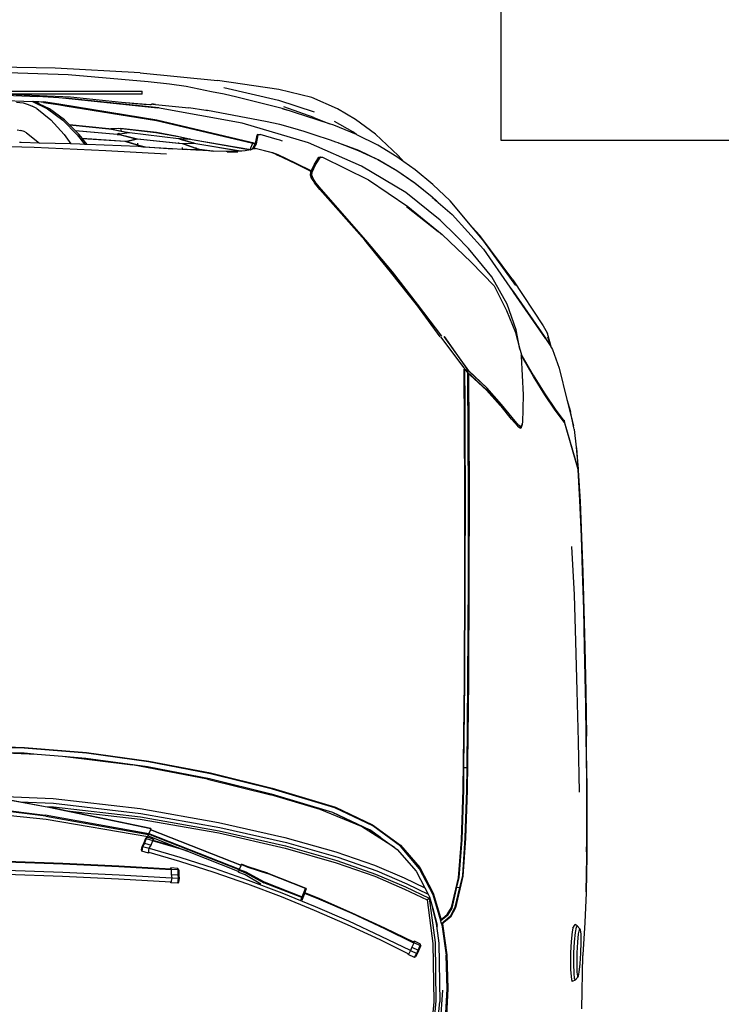
# Model space of a CAD drawing. Units: inches. Extents: x 0 to 4258, y 0 to 3769.
# Tile 14 of 30: x 3763 to 3796, y 3082 to 3128. Entities that reach past the tile are written whole.
import ezdxf

# ---------------------------------------------------------------- set-up
doc = ezdxf.new("R2010")
doc.units = ezdxf.units.IN
doc.header["$MEASUREMENT"] = 0
doc.layers.get('0').update_dxf_attribs({"color": 16})
doc.layers.add('A-FLOR-STRS', color=150, linetype='Continuous', lineweight=25)
doc.layers.add('C-PKNG-VEHI', color=8, linetype='Continuous', lineweight=18)
doc.layers.add('Edges', color=250, linetype='Continuous')

# ---------------------------------------------------------------- blocks, each defined once
blk = doc.blocks.new('Nissan Qashqai pl')
at = {"layer": 'Edges'}
for p, q in [((8.016, 12.8189), (7.9658, 12.8172)), ((7.9668, 12.8174), (8.0168, 12.8191)), ((8.0713, 12.8205), (8.016, 12.8189)), ((8.0168, 12.8191), (8.0718, 12.8207)), ((8.1249, 12.8218), (8.0713, 12.8205)), ((8.0718, 12.8207), (8.1251, 12.822)), ((8.1901, 12.8232), (8.1249, 12.8218)), ((8.1251, 12.822), (8.1902, 12.8233)), ((8.2094, 12.8235), (8.1901, 12.8232)), ((8.1902, 12.8233), (8.2543, 12.8243)), ((8.2543, 12.8243), (8.2094, 12.8235)), ((8.2543, 12.8243), (8.2094, 12.8235)), ((8.2544, 12.8242), (8.2094, 12.8235)), ((8.2693, 12.8245), (8.2543, 12.8243)), ((8.3166, 12.8249), (8.2544, 12.8242)), ((8.3098, 12.825), (8.2693, 12.8245)), ((8.3159, 12.825), (8.2693, 12.8245)), ((8.3159, 12.825), (8.3098, 12.825)), ((8.3159, 12.825), (8.3163, 12.825)), ((8.3163, 12.825), (8.3657, 12.8252)), ((8.3163, 12.825), (8.3597, 12.8252)), ((8.3764, 12.8251), (8.3166, 12.8249)), ((8.3597, 12.8252), (8.3657, 12.8252)), ((8.3657, 12.8252), (8.3663, 12.8252)), ((8.3663, 12.8252), (8.3747, 12.8252)), ((8.3764, 12.8251), (8.3663, 12.8252)), ((8.3747, 12.8252), (8.3757, 12.8252)), ((8.3757, 12.8252), (8.4282, 12.8249)), ((8.4069, 12.8249), (8.3764, 12.8251)), ((8.4219, 12.8246), (8.4069, 12.8249)), ((8.4292, 12.8248), (8.4069, 12.8249)), ((8.4282, 12.8249), (8.4799, 12.8239)), ((8.4799, 12.8239), (8.4292, 12.8248)), ((8.4799, 12.8239), (8.4811, 12.8239)), ((8.4811, 12.8239), (8.5241, 12.8222)), ((8.5241, 12.8222), (8.5707, 12.8193)), ((8.5707, 12.8193), (8.5719, 12.8193)), ((8.6489, 12.8179), (8.5719, 12.8193)), ((7.7673, 12.7961), (7.8058, 12.8055)), ((7.8087, 12.8062), (7.7848, 12.8012)), ((7.7936, 12.8029), (7.7977, 12.8038)), ((7.8676, 12.8123), (7.7998, 12.7928)), ((7.8012, 12.7929), (7.8681, 12.8121)), ((7.8106, 12.8065), (7.8087, 12.8062)), ((7.8106, 12.8065), (7.8107, 12.8065)), ((7.8107, 12.8065), (7.8363, 12.8097)), ((7.8363, 12.8097), (7.8676, 12.8123)), ((7.8363, 12.8097), (7.8381, 12.81)), ((7.8381, 12.81), (7.87, 12.8126)), ((7.8676, 12.8123), (7.8681, 12.8121)), ((7.869, 12.8124), (7.8681, 12.8121)), ((7.9137, 12.815), (7.869, 12.8124)), ((7.87, 12.8126), (7.9151, 12.8152)), ((7.9658, 12.8172), (7.9137, 12.815)), ((7.9151, 12.8152), (7.9668, 12.8174)), ((7.9803, 12.803), (8.05, 12.8066)), ((8.05, 12.8066), (8.1176, 12.8087)), ((8.1176, 12.8087), (8.1888, 12.8107)), ((8.1888, 12.8107), (8.2622, 12.8125)), ((8.2622, 12.8125), (8.3356, 12.8141)), ((8.5287, 12.8112), (8.5269, 12.8082)), ((8.5322, 12.8047), (8.5269, 12.8082)), ((8.5287, 12.8112), (8.5331, 12.815)), ((8.5287, 12.8112), (8.531, 12.8095)), ((8.531, 12.8095), (8.5385, 12.8079)), ((8.5322, 12.8047), (8.5375, 12.8036)), ((8.5347, 12.8159), (8.5331, 12.815)), ((8.5331, 12.815), (8.5346, 12.8138)), ((8.5346, 12.8138), (8.5406, 12.8125)), ((8.5407, 12.8167), (8.5347, 12.8159)), ((8.5385, 12.8079), (8.5518, 12.8066)), ((8.5406, 12.8125), (8.5526, 12.8114)), ((8.5527, 12.8169), (8.5407, 12.8167)), ((8.5518, 12.8066), (8.568, 12.8059)), ((8.5526, 12.8114), (8.5681, 12.8107)), ((8.5682, 12.8164), (8.5527, 12.8169)), ((8.568, 12.8059), (8.5842, 12.8057)), ((8.5681, 12.8107), (8.5836, 12.8104)), ((8.5837, 12.8154), (8.5682, 12.8164)), ((8.5836, 12.8104), (8.5957, 12.8107)), ((8.5958, 12.8141), (8.5837, 12.8154)), ((8.5842, 12.8057), (8.5974, 12.8061)), ((8.5957, 12.8107), (8.6017, 12.8114)), ((8.6018, 12.8129), (8.5958, 12.8141)), ((8.5974, 12.8061), (8.6049, 12.8069)), ((8.6017, 12.8114), (8.6032, 12.8121)), ((8.6032, 12.8121), (8.6018, 12.8129)), ((8.6073, 12.808), (8.6032, 12.8121)), ((8.6049, 12.8069), (8.6073, 12.808)), ((8.6065, 12.8027), (8.6093, 12.804)), ((8.6073, 12.808), (8.6093, 12.804)), ((7.7223, 12.7851), (7.7673, 12.7961)), ((7.7673, 12.7961), (7.7848, 12.8012)), ((7.7814, 12.7791), (7.7991, 12.7923)), ((7.7984, 12.7909), (7.7828, 12.7793)), ((7.7835, 12.8007), (7.7835, 12.8007)), ((7.7865, 12.8013), (7.7866, 12.8013)), ((7.7976, 12.792), (7.7991, 12.7923)), ((7.8007, 12.7926), (7.7984, 12.7909)), ((7.7991, 12.7923), (7.7998, 12.7928)), ((7.7995, 12.7924), (7.8007, 12.7926)), ((7.8012, 12.7929), (7.8007, 12.7926)), ((8.5375, 12.8036), (8.5513, 12.8023)), ((8.5513, 12.8023), (8.5678, 12.8016)), ((8.5678, 12.8016), (8.5844, 12.8014)), ((8.5844, 12.8014), (8.5921, 12.8016)), ((8.5921, 12.8016), (8.6021, 12.8022)), ((8.6021, 12.8022), (8.6065, 12.8027)), ((7.6926, 12.7737), (7.6953, 12.7753)), ((7.6953, 12.7753), (7.7223, 12.7851)), ((7.7591, 12.7641), (7.7814, 12.7791)), ((7.7828, 12.7793), (7.7606, 12.7644)), ((7.5946, 12.718), (7.6608, 12.7617)), ((7.6113, 12.7186), (7.6759, 12.7633)), ((7.6799, 12.7658), (7.6125, 12.719)), ((7.6608, 12.7617), (7.6712, 12.7675)), ((7.6712, 12.7675), (7.6721, 12.7679)), ((7.6926, 12.7737), (7.6721, 12.7679)), ((7.6759, 12.7633), (7.6793, 12.7657)), ((7.6911, 12.7728), (7.6774, 12.7688)), ((7.6793, 12.7657), (7.6802, 12.766)), ((7.6799, 12.7658), (7.6802, 12.766)), ((7.6802, 12.766), (7.6809, 12.7664)), ((7.6809, 12.7664), (7.6911, 12.7728)), ((7.6911, 12.7728), (7.6926, 12.7737)), ((7.7325, 12.7476), (7.7591, 12.7641)), ((7.7606, 12.7644), (7.7341, 12.7478)), ((7.7038, 12.731), (7.7325, 12.7476)), ((7.7341, 12.7478), (7.7056, 12.7314)), ((7.7048, 12.7302), (7.7608, 12.7329)), ((7.7608, 12.7329), (7.8014, 12.7318)), ((7.7688, 12.7328), (7.7688, 12.734)), ((7.6024, 12.7221), (7.5387, 12.6759)), ((7.6051, 12.7139), (7.6113, 12.7186)), ((7.6118, 12.7186), (7.6111, 12.7181)), ((7.6125, 12.719), (7.6118, 12.7186)), ((7.667, 12.723), (7.6295, 12.7097)), ((7.6386, 12.7089), (7.6708, 12.7217)), ((7.6949, 12.7283), (7.667, 12.723)), ((7.6708, 12.7217), (7.6949, 12.7283)), ((7.6949, 12.7283), (7.701, 12.73)), ((7.701, 12.73), (7.7024, 12.7301)), ((7.7024, 12.7301), (7.7038, 12.731)), ((7.7024, 12.7301), (7.7034, 12.7301)), ((7.7056, 12.7314), (7.7034, 12.7301)), ((7.7034, 12.7301), (7.7048, 12.7302)), ((7.7058, 12.7308), (7.7048, 12.7302)), ((7.8045, 12.7263), (7.7938, 12.7171)), ((7.8062, 12.725), (7.7959, 12.7161)), ((7.8014, 12.7318), (7.8022, 12.7316)), ((7.8022, 12.7316), (7.8037, 12.7315)), ((7.8022, 12.7316), (7.8072, 12.73)), ((7.8037, 12.7315), (7.8096, 12.7294)), ((7.8072, 12.73), (7.8045, 12.7263)), ((7.8062, 12.725), (7.8087, 12.7283)), ((7.8066, 12.7254), (7.8062, 12.725)), ((7.8096, 12.7294), (7.8066, 12.7254)), ((7.8072, 12.73), (7.8087, 12.7283)), ((7.5946, 12.718), (7.5304, 12.6704)), ((7.5501, 12.6757), (7.6051, 12.7139)), ((7.6295, 12.7097), (7.59, 12.6877)), ((7.6032, 12.6908), (7.6386, 12.7089)), ((7.6051, 12.7139), (7.6111, 12.7181)), ((7.7938, 12.7171), (7.7748, 12.7018)), ((7.7959, 12.7161), (7.7772, 12.7011)), ((7.5687, 12.6579), (7.6032, 12.6908)), ((7.7748, 12.7018), (7.7507, 12.6803)), ((7.753, 12.6794), (7.776, 12.6999)), ((7.776, 12.6999), (7.7539, 12.68)), ((7.7772, 12.7011), (7.776, 12.6999)), ((7.5501, 12.6757), (7.5001, 12.6302)), ((7.5387, 12.6759), (7.5184, 12.6591)), ((7.59, 12.6877), (7.5492, 12.654)), ((7.7261, 12.6543), (7.7507, 12.6803)), ((7.753, 12.6794), (7.7281, 12.6524)), ((7.7507, 12.6803), (7.7286, 12.6561)), ((7.7539, 12.68), (7.7324, 12.6565)), ((7.5184, 12.6591), (7.5304, 12.6704)), ((7.5184, 12.6591), (7.4801, 12.6274)), ((7.5289, 12.6158), (7.5687, 12.6579)), ((7.5492, 12.654), (7.531, 12.6359)), ((7.7261, 12.6543), (7.6762, 12.6186)), ((7.6762, 12.6186), (7.7233, 12.6514)), ((7.6771, 12.6135), (7.7215, 12.6473)), ((7.7215, 12.6473), (7.7221, 12.6478)), ((7.7232, 12.6486), (7.7221, 12.6478)), ((7.7281, 12.6524), (7.7232, 12.6486)), ((7.7245, 12.6486), (7.7232, 12.6486)), ((7.7267, 12.6539), (7.7233, 12.6514)), ((7.7261, 12.6476), (7.7238, 12.6476)), ((7.7294, 12.6487), (7.7245, 12.6486)), ((7.7279, 12.6477), (7.7261, 12.6476)), ((7.7286, 12.6561), (7.7267, 12.6539)), ((7.8048, 12.6483), (7.7279, 12.6477)), ((7.7299, 12.6537), (7.7281, 12.6524)), ((7.7281, 12.6524), (7.7349, 12.6524)), ((7.731, 12.6487), (7.7294, 12.6487)), ((7.7324, 12.6565), (7.7299, 12.6537)), ((7.7299, 12.6537), (7.7334, 12.6537)), ((7.764, 12.6489), (7.731, 12.6487)), ((7.7334, 12.6537), (7.8083, 12.6544)), ((7.7349, 12.6524), (7.768, 12.6527)), ((7.7662, 12.6489), (7.764, 12.6489)), ((7.7811, 12.649), (7.7662, 12.6489)), ((7.768, 12.6527), (7.7692, 12.6527)), ((7.7692, 12.6527), (7.7844, 12.6528)), ((7.7822, 12.649), (7.7811, 12.649)), ((7.8057, 12.6491), (7.7822, 12.649)), ((7.7844, 12.6528), (7.8078, 12.653)), ((7.9014, 12.6487), (7.8048, 12.6483)), ((7.8233, 12.6492), (7.8057, 12.6491)), ((7.8078, 12.653), (7.8233, 12.6531)), ((7.8083, 12.6544), (7.904, 12.6547)), ((7.8233, 12.6531), (7.9036, 12.6534)), ((7.902, 12.6495), (7.8233, 12.6492)), ((8.0273, 12.6485), (7.9014, 12.6487)), ((8.0275, 12.6493), (7.902, 12.6495)), ((7.9036, 12.6534), (8.0275, 12.6533)), ((7.904, 12.6547), (8.0276, 12.6545)), ((8.1753, 12.6479), (8.0273, 12.6485)), ((8.0275, 12.6533), (8.1755, 12.6527)), ((8.1754, 12.6487), (8.0275, 12.6493)), ((8.0276, 12.6545), (8.1753, 12.6539)), ((8.1753, 12.6539), (8.3324, 12.6521)), ((8.3318, 12.6462), (8.1753, 12.6479)), ((8.3002, 12.6474), (8.1754, 12.6487)), ((8.1755, 12.6527), (8.3005, 12.6514)), ((8.3005, 12.6514), (8.3002, 12.6474)), ((8.332, 12.6471), (8.3002, 12.6474)), ((8.3005, 12.6514), (8.3324, 12.651)), ((8.3324, 12.6521), (8.4022, 12.6498)), ((8.3324, 12.651), (8.4014, 12.6488)), ((8.4014, 12.6488), (8.4559, 12.6451)), ((8.4022, 12.6498), (8.4571, 12.6459)), ((7.531, 12.6359), (7.5081, 12.6131)), ((7.531, 12.6359), (7.5301, 12.6353)), ((8.4049, 12.6437), (8.3318, 12.6462)), ((8.4042, 12.6447), (8.332, 12.6471)), ((8.4588, 12.6405), (8.4042, 12.6447)), ((8.4595, 12.6395), (8.4049, 12.6437)), ((8.4559, 12.6451), (8.4736, 12.6409)), ((8.4571, 12.6459), (8.5029, 12.635)), ((8.4729, 12.6372), (8.4588, 12.6405)), ((8.5025, 12.6293), (8.4595, 12.6395)), ((8.4729, 12.6372), (8.4736, 12.6409)), ((8.5032, 12.6301), (8.4729, 12.6372)), ((8.4736, 12.6409), (8.5018, 12.6344)), ((8.5018, 12.6344), (8.5155, 12.6274)), ((8.5029, 12.635), (8.5163, 12.6279)), ((7.4801, 12.6274), (7.4565, 12.6023)), ((7.4827, 12.6103), (7.5001, 12.6302)), ((8.5125, 12.6231), (8.5025, 12.6293)), ((8.5132, 12.624), (8.5032, 12.6301)), ((8.5177, 12.617), (8.5125, 12.6231)), ((8.5132, 12.624), (8.5216, 12.6139)), ((8.5155, 12.6274), (8.5258, 12.6151)), ((8.5163, 12.6279), (8.5237, 12.6189)), ((8.5237, 12.6189), (8.5259, 12.6162)), ((8.5294, 12.6167), (8.5706, 12.6226)), ((8.5304, 12.6157), (8.5715, 12.6215)), ((8.5706, 12.6226), (8.6197, 12.6241)), ((8.6203, 12.6229), (8.5715, 12.6215)), ((8.6197, 12.6241), (8.6683, 12.6215)), ((8.6203, 12.6229), (8.6204, 12.6229)), ((8.6721, 12.6201), (8.6204, 12.6229)), ((7.5081, 12.6131), (7.4679, 12.5634)), ((7.4744, 12.6015), (7.4804, 12.6079)), ((7.4762, 12.6028), (7.478, 12.6049)), ((7.4804, 12.6079), (7.478, 12.6049)), ((7.478, 12.6049), (7.479, 12.6061)), ((7.479, 12.6061), (7.4815, 12.6089)), ((7.479, 12.6061), (7.4801, 12.6074)), ((7.4801, 12.6074), (7.4804, 12.6079)), ((7.4804, 12.6079), (7.4807, 12.6082)), ((7.4804, 12.6079), (7.4804, 12.6079)), ((7.4807, 12.6082), (7.4821, 12.6097)), ((7.4815, 12.6089), (7.4821, 12.6097)), ((7.4821, 12.6097), (7.4827, 12.6103)), ((7.4882, 12.5645), (7.5243, 12.6101)), ((7.4884, 12.5664), (7.5289, 12.6158)), ((7.5243, 12.6101), (7.5286, 12.6146)), ((7.676, 12.6152), (7.6296, 12.5803)), ((7.6769, 12.6129), (7.6306, 12.5791)), ((8.4814, 12.6029), (8.5166, 12.6135)), ((8.5216, 12.6139), (8.4838, 12.6027)), ((8.4889, 12.5969), (8.5531, 12.6055)), ((8.5039, 12.6023), (8.528, 12.6088)), ((8.5216, 12.6068), (8.5039, 12.6023)), ((8.5166, 12.6135), (8.5197, 12.6145)), ((8.5197, 12.6145), (8.5177, 12.617)), ((8.5197, 12.6145), (8.5216, 12.6139)), ((8.5258, 12.6151), (8.5216, 12.6139)), ((8.5216, 12.6068), (8.5538, 12.6111)), ((8.5301, 12.609), (8.5216, 12.6068)), ((8.5259, 12.6162), (8.5258, 12.6151)), ((8.5258, 12.6151), (8.5304, 12.6157)), ((8.5259, 12.6162), (8.5294, 12.6167)), ((8.5304, 12.6157), (8.5304, 12.6157)), ((8.5531, 12.6055), (8.6375, 12.6066)), ((8.5538, 12.6111), (8.6387, 12.6123)), ((8.622, 12.6161), (8.6699, 12.6132)), ((8.6375, 12.6066), (8.7481, 12.5968)), ((8.6721, 12.6093), (8.6387, 12.6123)), ((7.4565, 12.6023), (7.4354, 12.5766)), ((7.4542, 12.5765), (7.4744, 12.6015)), ((7.475, 12.6016), (7.4549, 12.5767)), ((7.4762, 12.6028), (7.475, 12.6016)), ((7.4752, 12.6016), (7.4762, 12.6028)), ((8.4444, 12.5834), (8.4814, 12.6029)), ((8.4838, 12.6027), (8.4462, 12.5833)), ((8.4499, 12.5782), (8.4737, 12.5908)), ((8.4594, 12.5611), (8.4737, 12.5908)), ((8.468, 12.5648), (8.4831, 12.5957)), ((8.4725, 12.563), (8.4889, 12.5969)), ((8.4737, 12.5908), (8.4831, 12.5957)), ((8.4756, 12.5615), (8.4914, 12.5942)), ((8.4831, 12.5957), (8.4867, 12.5977)), ((8.4867, 12.5977), (8.5039, 12.6023)), ((8.4914, 12.5942), (8.4889, 12.5969)), ((8.4914, 12.5942), (8.5544, 12.6026)), ((8.5544, 12.6026), (8.6386, 12.6037)), ((8.6386, 12.6037), (8.7491, 12.594)), ((7.4354, 12.5766), (7.4239, 12.5604)), ((7.4363, 12.5502), (7.4542, 12.5765)), ((7.4549, 12.5767), (7.4369, 12.5504)), ((7.6296, 12.5803), (7.5827, 12.5441)), ((7.6301, 12.5787), (7.618, 12.5691)), ((7.6306, 12.5791), (7.6301, 12.5787)), ((8.4122, 12.5558), (8.4444, 12.5834)), ((8.4462, 12.5833), (8.4134, 12.5554)), ((8.4183, 12.5508), (8.4499, 12.5782)), ((8.5554, 12.5847), (8.551, 12.5757)), ((8.5529, 12.5751), (8.5572, 12.5841)), ((8.5574, 12.5849), (8.5554, 12.5847)), ((8.5572, 12.5841), (8.5554, 12.5847)), ((8.5639, 12.581), (8.5572, 12.5841)), ((8.5574, 12.5849), (8.5584, 12.5846)), ((8.5582, 12.5845), (8.5574, 12.5849)), ((8.5584, 12.5846), (8.5649, 12.5816)), ((8.5595, 12.572), (8.5639, 12.581)), ((8.5687, 12.5791), (8.5639, 12.581)), ((8.5644, 12.5701), (8.5687, 12.5791)), ((8.5649, 12.5816), (8.5693, 12.5799)), ((8.5687, 12.5791), (8.5693, 12.5799)), ((8.5749, 12.5757), (8.5687, 12.5791)), ((8.5693, 12.5799), (8.5739, 12.5774)), ((8.5739, 12.5774), (8.5749, 12.5757)), ((7.4679, 12.5634), (7.4302, 12.4993)), ((7.4498, 12.5093), (7.4884, 12.5664)), ((7.618, 12.5691), (7.5829, 12.5411)), ((7.618, 12.5691), (7.584, 12.5429)), ((8.4493, 12.5212), (8.468, 12.5648)), ((8.454, 12.5196), (8.4725, 12.563)), ((8.5527, 12.5749), (8.5323, 12.5332)), ((8.5537, 12.5747), (8.5332, 12.5329)), ((8.5647, 12.57), (8.5441, 12.5279)), ((8.5487, 12.5256), (8.5692, 12.5674)), ((8.5527, 12.5749), (8.551, 12.5757)), ((8.551, 12.5757), (8.5528, 12.5751)), ((8.5528, 12.5751), (8.5527, 12.5749)), ((8.5528, 12.5751), (8.5529, 12.5751)), ((8.5529, 12.5751), (8.5537, 12.5747)), ((8.5537, 12.5747), (8.5595, 12.572)), ((8.5595, 12.572), (8.5644, 12.5701)), ((8.5644, 12.5701), (8.5647, 12.57)), ((8.5647, 12.57), (8.5692, 12.5675)), ((8.5692, 12.5674), (8.5692, 12.5675)), ((8.5692, 12.5675), (8.5705, 12.5668)), ((8.5705, 12.5668), (8.5692, 12.5674)), ((8.5749, 12.5757), (8.5705, 12.5668)), ((7.4147, 12.5524), (7.3837, 12.5197)), ((7.4166, 12.5503), (7.3997, 12.5227)), ((7.4239, 12.5604), (7.4147, 12.5524)), ((7.4239, 12.5604), (7.4166, 12.5503)), ((7.4205, 12.5229), (7.4363, 12.5502)), ((7.4369, 12.5504), (7.4211, 12.5232)), ((8.3826, 12.5151), (8.4122, 12.5558)), ((8.4134, 12.5554), (8.3844, 12.5157)), ((8.4156, 12.547), (8.4183, 12.5508)), ((8.4411, 12.5178), (8.4594, 12.5611)), ((8.4571, 12.5184), (8.4756, 12.5615)), ((7.5827, 12.5441), (7.5369, 12.5057)), ((7.584, 12.5429), (7.5568, 12.5201)), ((7.5829, 12.5411), (7.5568, 12.5201)), ((8.4154, 12.5468), (8.3852, 12.4994)), ((8.3901, 12.5113), (8.4154, 12.5468)), ((8.4011, 12.5269), (8.4154, 12.5468)), ((8.4156, 12.547), (8.4154, 12.5468)), ((8.5323, 12.5332), (8.5103, 12.4859)), ((7.3837, 12.5197), (7.3624, 12.4907)), ((7.3997, 12.5227), (7.3845, 12.4925)), ((7.4071, 12.4948), (7.4205, 12.5229)), ((7.4211, 12.5232), (7.4078, 12.4951)), ((7.5568, 12.5201), (7.5371, 12.5042)), ((8.4011, 12.5269), (8.3901, 12.5113)), ((8.3904, 12.512), (8.4011, 12.5269)), ((8.4296, 12.4651), (8.4493, 12.5212)), ((8.4343, 12.4637), (8.454, 12.5196)), ((8.5332, 12.5329), (8.5112, 12.4856)), ((8.5441, 12.5279), (8.5222, 12.4807)), ((8.5269, 12.4785), (8.5487, 12.5256)), ((7.4172, 12.4431), (7.4498, 12.5093)), ((7.5369, 12.5057), (7.4635, 12.4408)), ((8.3573, 12.4618), (8.3826, 12.5151)), ((8.3844, 12.5157), (8.3582, 12.4606)), ((8.3646, 12.4572), (8.39, 12.5111)), ((8.3648, 12.4579), (8.39, 12.5111)), ((8.39, 12.5111), (8.3852, 12.4994)), ((8.39, 12.5111), (8.3901, 12.5113)), ((8.3901, 12.5113), (8.3904, 12.512)), ((8.4217, 12.4622), (8.4411, 12.5178)), ((8.4375, 12.4627), (8.4571, 12.5184)), ((7.3624, 12.4907), (7.347, 12.4644)), ((7.3843, 12.492), (7.3707, 12.4592)), ((7.3843, 12.492), (7.3805, 12.4866)), ((7.3845, 12.4925), (7.3843, 12.492)), ((7.3962, 12.466), (7.4071, 12.4948)), ((7.4302, 12.4993), (7.3963, 12.4227)), ((7.4078, 12.4951), (7.3969, 12.4665)), ((7.4638, 12.439), (7.5371, 12.5042)), ((8.3852, 12.4994), (8.3608, 12.4393)), ((7.3805, 12.4866), (7.3655, 12.4604)), ((8.5103, 12.4859), (8.4895, 12.4381)), ((8.5112, 12.4856), (8.4904, 12.4377)), ((8.5222, 12.4807), (8.5014, 12.4329)), ((8.5062, 12.431), (8.5269, 12.4785)), ((7.347, 12.4644), (7.3309, 12.4276)), ((7.3951, 12.462), (7.3938, 12.4583)), ((7.3965, 12.4655), (7.3951, 12.462)), ((7.3965, 12.4655), (7.3962, 12.466)), ((7.3969, 12.4665), (7.3965, 12.4655)), ((7.3968, 12.4649), (7.3967, 12.4651)), ((8.4009, 12.3883), (8.4217, 12.4622)), ((8.4084, 12.3907), (8.4296, 12.4651)), ((8.4133, 12.3896), (8.4343, 12.4637)), ((8.4165, 12.3888), (8.4375, 12.4627)), ((7.3688, 12.4532), (7.3467, 12.3846)), ((7.3596, 12.4302), (7.3688, 12.4532)), ((7.3707, 12.4592), (7.3688, 12.4532)), ((7.3925, 12.4542), (7.3845, 12.4306)), ((7.3938, 12.4583), (7.3925, 12.4542)), ((8.3296, 12.3703), (8.3573, 12.4618)), ((8.3582, 12.4606), (8.3311, 12.3708)), ((8.3377, 12.3689), (8.3646, 12.4572)), ((8.3646, 12.4572), (8.3648, 12.4579)), ((8.3648, 12.4579), (8.3648, 12.4579)), ((7.4167, 12.4393), (7.4169, 12.4406)), ((7.4167, 12.4393), (7.4172, 12.4395)), ((7.417, 12.4377), (7.4167, 12.4393)), ((7.4169, 12.4412), (7.4172, 12.4431)), ((7.4169, 12.4406), (7.4172, 12.4423)), ((7.4169, 12.4406), (7.4169, 12.4412)), ((7.4169, 12.4398), (7.4169, 12.4406)), ((7.4282, 12.4328), (7.4169, 12.4398)), ((7.4172, 12.4395), (7.4169, 12.4398)), ((7.4283, 12.4307), (7.417, 12.4377)), ((7.4172, 12.4423), (7.4174, 12.4429)), ((7.4183, 12.4382), (7.4172, 12.4395)), ((7.4175, 12.4429), (7.4174, 12.4429)), ((7.4183, 12.4382), (7.4296, 12.4312)), ((7.4635, 12.4408), (7.4541, 12.4333)), ((7.4638, 12.439), (7.4541, 12.4313)), ((8.3608, 12.4393), (8.3392, 12.3684)), ((8.3608, 12.4393), (8.3608, 12.4393)), ((8.4895, 12.4381), (8.4811, 12.4174)), ((8.4904, 12.4377), (8.482, 12.4171)), ((7.3309, 12.4276), (7.3193, 12.3797)), ((7.3345, 12.3793), (7.3514, 12.4308)), ((7.3596, 12.4302), (7.344, 12.3869)), ((7.3963, 12.4227), (7.3676, 12.3269)), ((7.3845, 12.4306), (7.3799, 12.4164)), ((7.4255, 12.4044), (7.4367, 12.4268)), ((7.4365, 12.4235), (7.4267, 12.4041)), ((7.4387, 12.428), (7.4282, 12.4328)), ((7.4359, 12.4272), (7.4283, 12.4307)), ((7.4383, 12.4272), (7.4296, 12.4312)), ((7.4367, 12.4268), (7.4359, 12.4272)), ((7.4378, 12.4261), (7.4365, 12.4235)), ((7.4365, 12.4235), (7.4365, 12.4235)), ((7.4367, 12.4268), (7.4383, 12.4272)), ((7.4379, 12.4263), (7.4378, 12.4261)), ((7.4379, 12.4263), (7.4383, 12.4272)), ((7.4379, 12.4263), (7.4389, 12.4269)), ((7.4384, 12.426), (7.4379, 12.4263)), ((7.4384, 12.426), (7.438, 12.4251)), ((7.4383, 12.4272), (7.4389, 12.4269)), ((7.4389, 12.4269), (7.4384, 12.426)), ((7.4387, 12.4259), (7.4384, 12.426)), ((7.4431, 12.4276), (7.4387, 12.428)), ((7.443, 12.4254), (7.4387, 12.4259)), ((7.44, 12.4264), (7.4389, 12.4269)), ((7.44, 12.4264), (7.4442, 12.4258)), ((7.4477, 12.427), (7.443, 12.4254)), ((7.4479, 12.4293), (7.4431, 12.4276)), ((7.4442, 12.4258), (7.4477, 12.427)), ((7.4477, 12.427), (7.4541, 12.4313)), ((7.4541, 12.4333), (7.4479, 12.4293)), ((8.4742, 12.4188), (8.4754, 12.4193)), ((8.4754, 12.4193), (8.4747, 12.4185)), ((8.4754, 12.4193), (8.4876, 12.4144)), ((8.4791, 12.4183), (8.4754, 12.4193)), ((8.5014, 12.4329), (8.4817, 12.3847)), ((8.4866, 12.3829), (8.5062, 12.431)), ((7.3799, 12.4164), (7.375, 12.4)), ((8.4526, 12.3639), (8.4742, 12.4188)), ((8.4747, 12.4185), (8.4532, 12.3636)), ((8.4654, 12.3587), (8.4869, 12.4136)), ((8.4881, 12.4131), (8.4666, 12.3582)), ((8.4747, 12.4185), (8.4742, 12.4188)), ((8.4869, 12.4136), (8.4747, 12.4185)), ((8.4811, 12.4174), (8.4791, 12.4183)), ((8.482, 12.4171), (8.4811, 12.4174)), ((8.4912, 12.4133), (8.482, 12.4171)), ((8.4869, 12.4136), (8.4876, 12.4144)), ((8.4881, 12.4131), (8.4869, 12.4136)), ((8.4876, 12.4144), (8.4912, 12.4133)), ((8.4876, 12.4144), (8.4881, 12.4131)), ((8.4914, 12.4121), (8.4881, 12.4131)), ((8.4913, 12.4133), (8.4912, 12.4133)), ((8.4913, 12.4132), (8.4913, 12.4133)), ((7.3467, 12.3846), (7.3489, 12.3925)), ((7.375, 12.4), (7.3699, 12.3813)), ((7.4131, 12.3783), (7.4255, 12.4044)), ((7.4267, 12.4041), (7.4139, 12.3778)), ((7.3193, 12.3797), (7.3059, 12.291)), ((7.3161, 12.3001), (7.3345, 12.3793)), ((7.3467, 12.3846), (7.33, 12.3192)), ((7.3699, 12.3813), (7.3653, 12.3604)), ((7.3913, 12.3774), (7.3844, 12.3526)), ((7.3913, 12.3774), (7.3914, 12.3775)), ((7.3925, 12.3813), (7.3914, 12.3775)), ((7.3937, 12.3851), (7.3925, 12.3813)), ((7.4115, 12.3746), (7.4131, 12.3783)), ((7.4139, 12.3778), (7.4122, 12.3742)), ((7.4133, 12.3759), (7.4142, 12.3776)), ((8.3792, 12.2926), (8.4009, 12.3883)), ((8.3864, 12.2945), (8.4084, 12.3907)), ((8.3913, 12.2935), (8.4133, 12.3896)), ((8.3945, 12.2929), (8.4165, 12.3888)), ((8.4817, 12.3847), (8.4633, 12.3359)), ((8.4683, 12.3345), (8.4866, 12.3829)), ((7.4033, 12.3435), (7.4101, 12.3708)), ((7.4108, 12.3703), (7.4042, 12.3435)), ((7.4101, 12.3708), (7.4115, 12.3746)), ((7.4122, 12.3742), (7.4108, 12.3703)), ((8.3076, 12.281), (8.3296, 12.3703)), ((8.3311, 12.3708), (8.3089, 12.2811)), ((8.3157, 12.2795), (8.3377, 12.3689)), ((8.3166, 12.2767), (8.3392, 12.3684)), ((8.4526, 12.3639), (8.4434, 12.3353)), ((8.4439, 12.335), (8.4532, 12.3636)), ((7.3653, 12.3604), (7.3497, 12.2767)), ((7.3841, 12.3485), (7.3844, 12.3526)), ((7.3846, 12.3495), (7.3841, 12.3485)), ((7.3841, 12.3485), (7.3853, 12.3483)), ((7.3846, 12.3495), (7.3976, 12.347)), ((7.3971, 12.3461), (7.3853, 12.3483)), ((8.4509, 12.3322), (8.4654, 12.3587)), ((8.4521, 12.3317), (8.4666, 12.3582)), ((8.4547, 12.3309), (8.4682, 12.3538)), ((7.3971, 12.3461), (7.3635, 12.2033)), ((7.364, 12.2029), (7.3968, 12.3424)), ((7.3916, 12.2547), (7.4062, 12.3389)), ((7.4065, 12.3392), (7.3917, 12.2547)), ((7.3968, 12.3424), (7.398, 12.3449)), ((7.4046, 12.3389), (7.3968, 12.3424)), ((7.3983, 12.3458), (7.3971, 12.3461)), ((7.3976, 12.347), (7.4026, 12.3439)), ((7.398, 12.3449), (7.3999, 12.344)), ((7.398, 12.3449), (7.4012, 12.3441)), ((7.4012, 12.3441), (7.3983, 12.3458)), ((7.3999, 12.344), (7.4051, 12.3415)), ((7.3999, 12.344), (7.4048, 12.3417)), ((7.4033, 12.3427), (7.4012, 12.3441)), ((7.4012, 12.3441), (7.4015, 12.344)), ((7.4015, 12.344), (7.4028, 12.3437)), ((7.4026, 12.3439), (7.4033, 12.3435)), ((7.4033, 12.3435), (7.4042, 12.3422)), ((7.4042, 12.3422), (7.4033, 12.3427)), ((7.4042, 12.3435), (7.404, 12.3429)), ((7.404, 12.3429), (7.4043, 12.3428)), ((7.404, 12.3429), (7.4043, 12.3425)), ((7.4041, 12.3435), (7.4042, 12.3435)), ((7.4042, 12.3435), (7.4045, 12.3434)), ((7.4042, 12.3422), (7.4043, 12.3425)), ((7.4044, 12.3422), (7.4042, 12.3422)), ((7.4043, 12.3428), (7.4045, 12.3434)), ((7.4043, 12.3428), (7.4046, 12.3425)), ((7.4043, 12.3425), (7.4043, 12.3428)), ((7.4043, 12.3425), (7.4044, 12.3422)), ((7.4044, 12.3422), (7.4046, 12.3419)), ((7.4046, 12.3422), (7.4044, 12.3422)), ((7.4045, 12.3434), (7.405, 12.3456)), ((7.4045, 12.3434), (7.4048, 12.3433)), ((7.4046, 12.3425), (7.4047, 12.3424)), ((7.4047, 12.3424), (7.4046, 12.3422)), ((7.4046, 12.3422), (7.4046, 12.3419)), ((7.4048, 12.3422), (7.4046, 12.3422)), ((7.4046, 12.3419), (7.405, 12.3419)), ((7.4048, 12.3417), (7.4046, 12.3419)), ((7.4046, 12.3389), (7.4062, 12.3389)), ((7.4047, 12.3424), (7.4048, 12.3422)), ((7.4048, 12.3422), (7.405, 12.3419)), ((7.4048, 12.3417), (7.4052, 12.3416)), ((7.4051, 12.3415), (7.4048, 12.3417)), ((7.405, 12.3419), (7.4052, 12.3416)), ((7.4051, 12.3415), (7.4052, 12.3415)), ((7.4052, 12.3416), (7.4052, 12.3415)), ((7.4052, 12.3415), (7.4063, 12.3395)), ((7.4062, 12.3389), (7.4063, 12.3395)), ((7.4063, 12.3395), (7.4065, 12.3392)), ((7.4065, 12.3392), (7.4066, 12.3389)), ((7.4066, 12.3389), (7.408, 12.3313)), ((8.4434, 12.3353), (8.4397, 12.326)), ((8.4403, 12.3257), (8.4439, 12.335)), ((8.4633, 12.3359), (8.4461, 12.2868)), ((8.4512, 12.2856), (8.4683, 12.3345)), ((7.3676, 12.3269), (7.3455, 12.2042)), ((7.3971, 12.2599), (7.4083, 12.3258)), ((7.4084, 12.3244), (7.3975, 12.2599)), ((7.408, 12.3313), (7.4083, 12.3258)), ((7.4083, 12.3258), (7.4084, 12.3244)), ((7.4084, 12.3244), (7.4087, 12.3195)), ((7.4087, 12.3195), (7.4087, 12.3037)), ((7.4092, 12.3184), (7.4091, 12.3206)), ((8.3894, 12.1944), (8.4409, 12.3255)), ((8.4415, 12.3252), (8.3899, 12.1941)), ((8.3951, 12.192), (8.4467, 12.3231)), ((8.4479, 12.3226), (8.3963, 12.1915)), ((8.4209, 12.2475), (8.4502, 12.3219)), ((8.4403, 12.3257), (8.4397, 12.326)), ((8.4409, 12.3255), (8.4403, 12.3257)), ((8.4415, 12.3252), (8.4409, 12.3255)), ((8.4467, 12.3231), (8.4415, 12.3252)), ((8.4472, 12.3229), (8.4467, 12.3231)), ((8.4472, 12.3229), (8.4509, 12.3322)), ((8.4479, 12.3226), (8.4472, 12.3229)), ((8.4484, 12.3224), (8.4479, 12.3226)), ((8.4484, 12.3224), (8.4521, 12.3317)), ((8.4502, 12.3219), (8.4484, 12.3224)), ((8.4511, 12.3216), (8.4502, 12.3219)), ((8.4511, 12.3216), (8.4547, 12.3309)), ((7.33, 12.3192), (7.3261, 12.3009)), ((7.4092, 12.305), (7.4092, 12.3184)), ((7.3261, 12.3009), (7.3223, 12.2825)), ((7.4087, 12.3037), (7.4081, 12.2848)), ((8.3593, 12.1791), (8.3792, 12.2926)), ((8.3662, 12.1803), (8.3864, 12.2945)), ((8.3713, 12.1796), (8.3913, 12.2935)), ((8.3745, 12.1792), (8.3945, 12.2929)), ((7.2951, 12.1791), (7.3059, 12.291)), ((7.3223, 12.2825), (7.3186, 12.2641)), ((7.3498, 12.2768), (7.3494, 12.2741)), ((7.4054, 12.2651), (7.4081, 12.2848)), ((7.4079, 12.2798), (7.4059, 12.2651)), ((7.4079, 12.2798), (7.4069, 12.2598)), ((7.4081, 12.2838), (7.4079, 12.2798)), ((7.4081, 12.2848), (7.4081, 12.2838)), ((8.2905, 12.1918), (8.3076, 12.281)), ((8.3089, 12.2811), (8.2916, 12.1913)), ((8.2985, 12.1901), (8.3157, 12.2795)), ((8.4461, 12.2868), (8.4302, 12.2373)), ((8.4353, 12.2363), (8.4512, 12.2856)), ((7.3186, 12.2641), (7.3149, 12.2457)), ((7.3494, 12.2741), (7.3457, 12.2495)), ((7.3497, 12.2767), (7.3494, 12.2741)), ((7.4038, 12.2599), (7.4049, 12.2631)), ((7.4049, 12.2631), (7.4054, 12.2651)), ((7.4059, 12.2651), (7.4058, 12.2632)), ((7.4058, 12.2632), (7.4059, 12.2618)), ((8.3166, 12.2767), (8.296, 12.168)), ((7.3407, 12.2016), (7.3457, 12.2495)), ((7.3909, 12.2508), (7.3864, 12.231)), ((7.3869, 12.2347), (7.3912, 12.2527)), ((7.3901, 12.2368), (7.391, 12.2507)), ((7.3914, 12.2527), (7.3906, 12.2386)), ((7.3908, 12.2366), (7.3965, 12.256)), ((7.3911, 12.2518), (7.3909, 12.2508)), ((7.391, 12.2387), (7.3967, 12.2579)), ((7.391, 12.2507), (7.3911, 12.2518)), ((7.3912, 12.2517), (7.3911, 12.2518)), ((7.3912, 12.2527), (7.3916, 12.2547)), ((7.3917, 12.2547), (7.3914, 12.2527)), ((7.3969, 12.257), (7.3965, 12.256)), ((7.3967, 12.2579), (7.3971, 12.2599)), ((7.3968, 12.2559), (7.3969, 12.257)), ((7.3972, 12.2421), (7.3968, 12.2559)), ((7.3975, 12.2599), (7.3973, 12.258)), ((7.3973, 12.258), (7.3977, 12.2439)), ((7.4048, 12.2612), (7.3982, 12.2419)), ((7.3983, 12.244), (7.4038, 12.2599)), ((7.4028, 12.2599), (7.4038, 12.2599)), ((7.4053, 12.2622), (7.4048, 12.2612)), ((7.4053, 12.2612), (7.4053, 12.2622)), ((7.4061, 12.2473), (7.4053, 12.2612)), ((7.4059, 12.2618), (7.4056, 12.2621)), ((7.4059, 12.2618), (7.4064, 12.2523)), ((7.4064, 12.2523), (7.4061, 12.2473)), ((7.4069, 12.2598), (7.4064, 12.2523)), ((7.3149, 12.2457), (7.3113, 12.2217)), ((7.3813, 12.2021), (7.3869, 12.2347)), ((7.3815, 12.1638), (7.3899, 12.2348)), ((7.3903, 12.2347), (7.382, 12.1639)), ((7.3899, 12.2348), (7.3901, 12.2368)), ((7.3908, 12.2366), (7.3903, 12.2347)), ((7.3905, 12.1754), (7.3966, 12.2347)), ((7.3906, 12.2386), (7.3907, 12.2376)), ((7.3907, 12.2376), (7.391, 12.2387)), ((7.3977, 12.24), (7.3911, 12.1755)), ((7.3957, 12.2348), (7.3966, 12.2348)), ((7.3957, 12.2347), (7.3966, 12.2347)), ((7.3966, 12.2348), (7.3972, 12.24)), ((7.3966, 12.2347), (7.3966, 12.2348)), ((7.3972, 12.24), (7.3972, 12.2421)), ((7.3977, 12.2439), (7.398, 12.2429)), ((7.3982, 12.2419), (7.3977, 12.24)), ((7.398, 12.2429), (7.3983, 12.244)), ((7.4032, 12.24), (7.4057, 12.24)), ((7.4057, 12.24), (7.4048, 12.2262)), ((7.4061, 12.2472), (7.4057, 12.24)), ((7.4061, 12.2472), (7.4061, 12.2473)), ((8.3986, 12.1908), (8.4163, 12.2359)), ((8.4163, 12.2359), (8.4052, 12.1979)), ((8.4191, 12.2418), (8.4061, 12.1973)), ((8.4163, 12.2359), (8.4209, 12.2475)), ((8.4302, 12.2373), (8.4171, 12.1926)), ((8.4209, 12.2475), (8.4191, 12.2418)), ((8.4224, 12.1919), (8.4353, 12.2363)), ((8.4475, 12.2348), (8.4457, 12.2337)), ((8.4476, 12.2341), (8.4457, 12.2337)), ((8.4471, 12.2242), (8.4476, 12.2341)), ((8.4475, 12.2348), (8.4484, 12.235)), ((8.4555, 12.2348), (8.4475, 12.2348)), ((8.4549, 12.2341), (8.4476, 12.2341)), ((8.4484, 12.235), (8.4557, 12.235)), ((8.4544, 12.2242), (8.4549, 12.2341)), ((8.46, 12.2348), (8.4549, 12.2341)), ((8.4557, 12.235), (8.4603, 12.2357)), ((8.4595, 12.2249), (8.46, 12.2348)), ((8.46, 12.2348), (8.4603, 12.2357)), ((8.4671, 12.2337), (8.46, 12.2348)), ((8.4603, 12.2357), (8.4655, 12.2348)), ((8.4655, 12.2348), (8.4671, 12.2337)), ((7.3113, 12.2217), (7.3078, 12.191)), ((7.3864, 12.231), (7.3815, 12.2029)), ((7.4022, 12.187), (7.4048, 12.2262)), ((7.4048, 12.2262), (7.4023, 12.1836)), ((8.4471, 12.2238), (8.4425, 12.1485)), ((8.448, 12.2241), (8.4435, 12.1487)), ((8.4457, 12.2337), (8.4452, 12.2238)), ((8.4452, 12.2238), (8.4471, 12.2242)), ((8.4471, 12.2238), (8.4452, 12.2238)), ((8.4471, 12.2242), (8.4544, 12.2242)), ((8.4471, 12.2239), (8.4471, 12.2238)), ((8.4544, 12.2242), (8.4595, 12.2249)), ((8.4601, 12.2247), (8.4555, 12.1488)), ((8.4595, 12.2249), (8.4666, 12.2237)), ((8.4607, 12.1481), (8.4652, 12.2237)), ((8.4652, 12.2237), (8.4652, 12.2238)), ((8.4666, 12.2237), (8.4652, 12.2237)), ((8.4671, 12.2337), (8.4666, 12.2237)), ((7.3455, 12.2062), (7.3317, 12.0717)), ((7.4072, 12.1299), (7.4124, 12.2176)), ((7.3317, 12.0717), (7.3455, 12.2042)), ((7.3407, 12.2016), (7.34, 12.1962)), ((7.34, 12.1962), (7.3401, 12.1962)), ((7.3401, 12.1962), (7.341, 12.1962)), ((7.3403, 12.1981), (7.3407, 12.2016)), ((7.3635, 12.2033), (7.3405, 12.0616)), ((7.3413, 12.1933), (7.3407, 12.1879)), ((7.341, 12.1962), (7.3414, 12.1962)), ((7.341, 12.1962), (7.341, 12.1962)), ((7.3414, 12.1962), (7.341, 12.1962)), ((7.341, 12.1962), (7.3413, 12.1933)), ((7.3413, 12.1931), (7.341, 12.1848)), ((7.3415, 12.1954), (7.3413, 12.1933)), ((7.3413, 12.1933), (7.3413, 12.1931)), ((7.3426, 12.0707), (7.364, 12.2029)), ((7.375, 12.1484), (7.3813, 12.2021)), ((7.3815, 12.2029), (7.3756, 12.1509)), ((8.2781, 12.1018), (8.2905, 12.1918)), ((8.3887, 12.1946), (8.3575, 12.0475)), ((8.3882, 12.1948), (8.3618, 12.07)), ((8.3957, 12.1917), (8.3688, 12.0419)), ((8.3887, 12.1946), (8.3882, 12.1948)), ((8.3882, 12.1948), (8.3894, 12.1944)), ((8.3894, 12.1944), (8.3887, 12.1946)), ((8.3894, 12.1944), (8.3894, 12.1944)), ((8.3894, 12.1944), (8.3899, 12.1941)), ((8.3899, 12.1941), (8.3951, 12.192)), ((8.3951, 12.192), (8.3963, 12.1915)), ((8.3957, 12.1917), (8.3951, 12.192)), ((8.3969, 12.1913), (8.3957, 12.1917)), ((8.3963, 12.1915), (8.3986, 12.1908)), ((8.4035, 12.1986), (8.4007, 12.189)), ((8.4023, 12.1879), (8.4052, 12.1975)), ((8.4052, 12.1975), (8.4035, 12.1986)), ((8.4035, 12.1986), (8.4052, 12.1979)), ((8.4052, 12.1979), (8.4052, 12.1978)), ((8.412, 12.195), (8.4052, 12.1975)), ((8.4092, 12.1855), (8.412, 12.195)), ((8.4167, 12.1925), (8.412, 12.195)), ((8.4139, 12.1829), (8.4167, 12.1925)), ((8.4237, 12.1914), (8.4167, 12.1925)), ((8.4237, 12.1914), (8.4209, 12.1819)), ((8.4223, 12.1918), (8.4224, 12.1919)), ((8.4224, 12.1919), (8.4237, 12.1914)), ((7.2951, 12.1791), (7.2884, 12.0562)), ((7.3078, 12.191), (7.298, 12.075)), ((7.3261, 12.1821), (7.3216, 12.1821)), ((7.3216, 11.6621), (7.3216, 12.1821)), ((7.3261, 12.1821), (7.3261, 11.9779)), ((7.3407, 12.1879), (7.3378, 12.1521)), ((7.341, 12.1848), (7.34, 12.1731)), ((7.4021, 12.1833), (7.3951, 12.1606)), ((7.399, 12.1756), (7.4017, 12.185)), ((7.4017, 12.185), (7.4022, 12.187)), ((7.4023, 12.1836), (7.4018, 12.1764)), ((7.4023, 12.1836), (7.4021, 12.1833)), ((8.2916, 12.1913), (8.2793, 12.1016)), ((8.2862, 12.1008), (8.2985, 12.1901)), ((8.3448, 12.0536), (8.3593, 12.1791)), ((8.3516, 12.0542), (8.3662, 12.1803)), ((8.3567, 12.0538), (8.3713, 12.1796)), ((8.3618, 12.07), (8.3745, 12.1792)), ((8.3702, 12.0427), (8.3969, 12.1913)), ((8.3746, 12.0435), (8.3995, 12.1905)), ((8.3995, 12.1905), (8.3969, 12.1913)), ((8.3995, 12.1905), (8.3986, 12.1908)), ((8.4007, 12.189), (8.4023, 12.1879)), ((8.4007, 12.189), (8.402, 12.1874)), ((8.4028, 12.1868), (8.402, 12.1874)), ((8.402, 12.1874), (8.4027, 12.1871)), ((8.4023, 12.1879), (8.4092, 12.1855)), ((8.4097, 12.1844), (8.4028, 12.1868)), ((8.4092, 12.1855), (8.4139, 12.1829)), ((8.4139, 12.1821), (8.4097, 12.1844)), ((8.4139, 12.1829), (8.4209, 12.1819)), ((8.4139, 12.1821), (8.4139, 12.1829)), ((8.4191, 12.1813), (8.4139, 12.1821)), ((8.4209, 12.1819), (8.4191, 12.1813)), ((7.34, 12.1731), (7.3378, 12.1521)), ((7.3812, 12.1619), (7.3815, 12.1638)), ((7.382, 12.1639), (7.382, 12.1619)), ((7.3843, 12.1498), (7.3877, 12.1639)), ((7.3903, 12.1716), (7.3844, 12.1479)), ((7.3877, 12.1639), (7.3874, 12.1639)), ((7.3877, 12.1639), (7.3901, 12.1734)), ((7.3901, 12.1734), (7.3905, 12.1754)), ((7.3907, 12.1727), (7.3903, 12.1716)), ((7.3909, 12.1716), (7.3907, 12.1727)), ((7.3939, 12.1596), (7.3909, 12.1716)), ((7.3911, 12.1755), (7.3913, 12.1737)), ((7.3913, 12.1737), (7.3943, 12.1614)), ((7.3949, 12.1616), (7.399, 12.1756)), ((7.3967, 12.1756), (7.399, 12.1756)), ((7.4018, 12.1764), (7.3986, 12.1025)), ((8.2834, 12.0669), (8.296, 12.168)), ((7.3378, 12.1521), (7.3302, 12.0785)), ((7.3756, 12.1509), (7.3792, 12.1518)), ((7.3756, 12.1509), (7.3762, 12.138)), ((7.3813, 12.1599), (7.3763, 12.1361)), ((7.3764, 12.138), (7.3792, 12.1518)), ((7.3792, 12.1518), (7.3812, 12.1619)), ((7.3815, 12.161), (7.3813, 12.1599)), ((7.3817, 12.16), (7.3815, 12.161)), ((7.3832, 12.1493), (7.3817, 12.16)), ((7.382, 12.1619), (7.3838, 12.1497)), ((7.3832, 12.1493), (7.3824, 12.1487)), ((7.3824, 12.1487), (7.3832, 12.1492)), ((7.3836, 12.1459), (7.3824, 12.1487)), ((7.3824, 12.1487), (7.3835, 12.1468)), ((7.3838, 12.1497), (7.3832, 12.1493)), ((7.3832, 12.1492), (7.3837, 12.1495)), ((7.3832, 12.1492), (7.3832, 12.1493)), ((7.3837, 12.1495), (7.3843, 12.1498)), ((7.3837, 12.1495), (7.3838, 12.1497)), ((7.384, 12.1459), (7.3842, 12.1495)), ((7.3842, 12.1495), (7.3843, 12.1498)), ((7.3843, 12.1495), (7.3842, 12.1495)), ((7.3896, 12.0954), (7.3941, 12.1576)), ((7.3945, 12.1577), (7.3903, 12.0959)), ((7.3941, 12.1576), (7.3939, 12.1596)), ((7.3943, 12.1614), (7.3947, 12.1605)), ((7.3951, 12.1606), (7.3945, 12.1577)), ((7.3947, 12.1605), (7.3949, 12.1616)), ((8.4435, 12.1487), (8.4397, 12.0674)), ((8.4555, 12.1488), (8.4517, 12.0674)), ((7.376, 12.136), (7.375, 12.1484)), ((7.3759, 12.1341), (7.376, 12.136)), ((7.3763, 12.1361), (7.3761, 12.1341)), ((7.3762, 12.137), (7.3764, 12.138)), ((7.3762, 12.138), (7.3762, 12.137)), ((7.3764, 12.1371), (7.3762, 12.137)), ((7.3783, 12.0852), (7.3836, 12.1459)), ((7.384, 12.1459), (7.3788, 12.0857)), ((7.3836, 12.1459), (7.3835, 12.1468)), ((7.3835, 12.1468), (7.384, 12.1459)), ((7.3844, 12.1479), (7.384, 12.1459)), ((8.4425, 12.1485), (8.4387, 12.0674)), ((8.4568, 12.0669), (8.4607, 12.1481)), ((7.3701, 12.0771), (7.3759, 12.1341)), ((7.3761, 12.1341), (7.3704, 12.0773)), ((7.4025, 12.026), (7.4072, 12.1299)), ((7.3896, 12.0954), (7.3841, 12.091)), ((7.3845, 12.0883), (7.3985, 12.0993)), ((7.3903, 12.0959), (7.3896, 12.0954)), ((7.3986, 12.1025), (7.3903, 12.0959)), ((7.3982, 12.092), (7.3978, 12.0791)), ((7.3985, 12.0993), (7.3982, 12.092)), ((7.3986, 12.1025), (7.3985, 12.0993)), ((8.2708, 12.0123), (8.2781, 12.1018)), ((8.2793, 12.1016), (8.2719, 12.0118)), ((8.2834, 12.0669), (8.2862, 12.1008)), ((7.3302, 12.0785), (7.3261, 11.9779)), ((7.3633, 12.0674), (7.3845, 12.0883)), ((7.3783, 12.0852), (7.3704, 12.0773)), ((7.3788, 12.0857), (7.3783, 12.0852)), ((7.3841, 12.091), (7.3788, 12.0857)), ((7.3842, 12.0693), (7.3978, 12.0791)), ((7.3978, 12.0791), (7.3966, 12.0338)), ((7.298, 12.075), (7.2928, 11.9221)), ((7.3309, 12.0619), (7.3317, 12.0717)), ((7.341, 12.0605), (7.3426, 12.0707)), ((7.3631, 12.0701), (7.3469, 12.0481)), ((7.3471, 12.0454), (7.3633, 12.0674)), ((7.363, 12.0501), (7.3842, 12.0693)), ((7.3701, 12.0771), (7.3631, 12.0701)), ((7.3704, 12.0773), (7.3701, 12.0771)), ((8.2804, 12.0305), (8.2834, 12.0669)), ((8.3618, 12.07), (8.3574, 12.0489)), ((8.4387, 12.0674), (8.4359, 11.9861)), ((8.4397, 12.0674), (8.4369, 11.9861)), ((8.4517, 12.0674), (8.4489, 11.9858)), ((8.4541, 11.9857), (8.4568, 12.0669)), ((7.2884, 12.0562), (7.2857, 11.9221)), ((7.3294, 12.0385), (7.3309, 12.0619)), ((7.3405, 12.0616), (7.3369, 12.0394)), ((7.3377, 12.0398), (7.341, 12.0605)), ((7.3468, 12.0299), (7.363, 12.0501)), ((8.3406, 11.9567), (8.3448, 12.0536)), ((8.3495, 12.0053), (8.3516, 12.0542)), ((8.3562, 12.0421), (8.3567, 12.0538)), ((7.3294, 12.0385), (7.3291, 12.0316)), ((7.3365, 12.0237), (7.3471, 12.0454)), ((7.3365, 12.0321), (7.3369, 12.0394)), ((7.3377, 12.0398), (7.3369, 12.0328)), ((7.3469, 12.0481), (7.3402, 12.0337)), ((8.3575, 12.0475), (8.3104, 11.7881)), ((8.336, 11.7828), (8.3688, 12.0419)), ((8.3702, 12.0427), (8.3374, 11.7826)), ((8.3495, 12.0053), (8.3562, 12.0421)), ((8.3562, 12.0421), (8.3574, 12.0489)), ((8.3565, 11.8707), (8.3746, 12.0435)), ((7.3251, 11.9221), (7.3291, 12.0316)), ((7.3329, 11.9221), (7.3365, 12.0237)), ((7.3362, 12.0248), (7.3365, 12.0321)), ((7.3362, 12.0248), (7.3366, 12.0246)), ((7.3365, 12.0237), (7.3362, 12.0248)), ((7.3369, 12.0287), (7.3369, 12.0328)), ((7.338, 12.0291), (7.3369, 12.0287)), ((7.3374, 12.0276), (7.3369, 12.0287)), ((7.338, 12.0291), (7.3374, 12.0276)), ((7.3402, 12.0337), (7.338, 12.0291)), ((7.3387, 12.0332), (7.3402, 12.0337)), ((7.3407, 12.0176), (7.3432, 12.0231)), ((7.3468, 12.0299), (7.3432, 12.0231)), ((7.3818, 12.0151), (7.3966, 12.0338)), ((7.3966, 12.0338), (7.3959, 12.0071)), ((7.4002, 11.9221), (7.4025, 12.026)), ((8.2765, 11.9273), (8.2804, 12.0305)), ((8.2788, 12.0114), (8.2804, 12.0305)), ((7.3373, 12.0004), (7.3386, 12.01)), ((7.3386, 12.01), (7.3407, 12.0176)), ((7.3775, 12.0015), (7.3786, 12.007)), ((7.3801, 12.0115), (7.3786, 12.007)), ((7.3818, 12.0151), (7.3801, 12.0115)), ((7.3959, 12.0071), (7.3959, 12.0051)), ((8.2682, 11.9221), (8.2708, 12.0123)), ((8.2719, 12.0118), (8.2695, 11.9221)), ((8.2765, 11.9273), (8.2788, 12.0114)), ((8.3406, 11.9567), (8.3495, 12.0053))]:
    blk.add_line(p, q, dxfattribs=at)
blk = doc.blocks.new('car')
blk.add_blockref('Nissan Qashqai pl', (-9.7433, -11.9151))

msp = doc.modelspace()

# ---------------------------------------------------------------- linework, layer by layer
at = {"layer": 'A-FLOR-STRS'}
for p, q in [((3786.102, 3122.34), (3786.102, 3163.293)), ((3828.116, 3122.34), (3786.102, 3122.34))]:
    msp.add_line(p, q, dxfattribs=at)

# ---------------------------------------------------------------- block references
at = {"layer": 'C-PKNG-VEHI', "xscale": 32.66500240257601, "yscale": 32.66500240257601, "zscale": 32.66500240257601, "rotation": 270}
msp.add_blockref('car', (3760.419, 3045.57), dxfattribs=at)

doc.saveas('drawing.dxf')
